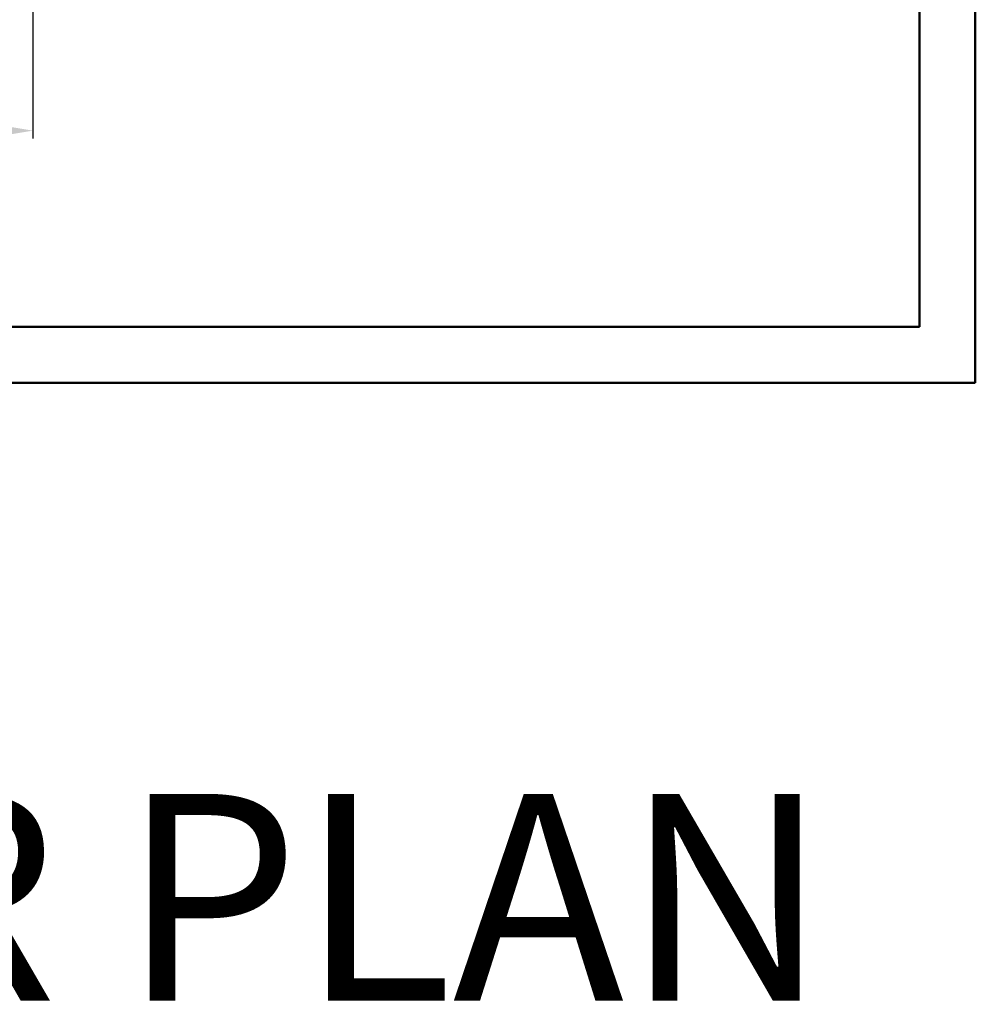
# Model space of a CAD drawing. Units: inches. Extents: x 116541 to 117938, y 135634 to 136328.
# Tile 6 of 9: x 117747 to 117902, y 135634 to 135793. Entities that reach past the tile are written whole.
import ezdxf

# ---------------------------------------------------------------- set-up
doc = ezdxf.new("R2010")
doc.units = ezdxf.units.IN
for name, color, linetype, lineweight in [('A-ANNO-DIMS', 2, 'Continuous', 18), ('A-ANNO-TEXT', 7, 'Continuous', 25), ('A-WALL', 7, 'Continuous', 50)]:
    doc.layers.add(name, color=color, linetype=linetype, lineweight=lineweight)
doc.styles.get("Standard").update_dxf_attribs({"font": 'arial.ttf'})
doc.dimstyles.new('ISO-25', dxfattribs={"dimtxt": 5, "dimasz": 4, "dimexe": 1.25, "dimexo": 0.625, "dimtad": 1, "dimdec": 3, "dimlunit": 3, "dimtxsty": 'Standard', "dimcen": 2.5, "dimadec": 0, "dimazin": 0, "dimtfac": 1, "dimtdec": 3, "dimtmove": 0, "dimatfit": 3, "dimfxl": 1, "dimarcsym": 0})

# ---------------------------------------------------------------- blocks, each defined once
blk = doc.blocks.new('*D50')
at = {"layer": 'A-ANNO-DIMS', "color": 0, "lineweight": -2, "transparency": 16777216}
for p, q in [((117487.52, 135796.88), (117487.52, 135773.9)), ((117749.52, 135796.88), (117749.52, 135773.9)), ((117491.52, 135775.15), (117745.52, 135775.15))]:
    blk.add_line(p, q, dxfattribs=at)
at = {"layer": 'A-ANNO-DIMS', "color": 0, "transparency": 16777216}
for points in [[(117491.52, 135775.82), (117491.52, 135774.49), (117487.52, 135775.15)], [(117745.52, 135775.82), (117745.52, 135774.49), (117749.52, 135775.15)]]:
    blk.add_solid(points, dxfattribs=at)
at = {"layer": 'Defpoints', "color": 0, "transparency": 16777216}
for p in [(117487.52, 135797.5), (117749.52, 135797.5), (117749.52, 135775.15)]:
    blk.add_point(p, dxfattribs=at)
at = {"layer": 'A-ANNO-DIMS', "color": 0, "transparency": 16777216, "insert": (117618.52, 135778.33), "char_height": 5, "attachment_point": 5}
blk.add_mtext('21\'-10"', dxfattribs=at)

msp = doc.modelspace()

# ---------------------------------------------------------------- linework, layer by layer
at = {"layer": 'A-WALL'}
for p, q in [((117901.5209, 136286.5034), (117901.5209, 135734.5034)), ((117892.5209, 136244.5034), (117892.5209, 135750.0323)), ((117892.5209, 135743.5034), (117892.5209, 135750.0323)), ((117698.4977, 135743.5034), (117892.5209, 135743.5034)), ((117454.5209, 135734.5034), (117871.5209, 135734.5034)), ((117871.5209, 135734.5034), (117901.5209, 135734.5034))]:
    msp.add_line(p, q, dxfattribs=at)

# ---------------------------------------------------------------- texts
at = {"layer": 'A-ANNO-TEXT'}
msp.add_text('FIRST FLOOR PLAN', height=33.340721, dxfattribs=at).set_placement((117475.5022, 135634.8462))

# ---------------------------------------------------------------- dimensions: what is measured, and where the dimension line sits
at = {"layer": 'A-ANNO-DIMS'}
dim = msp.add_linear_dim(base=(117749.5209, 135775.1534), p1=(117487.5209, 135797.5034), p2=(117749.5209, 135797.5034), dimstyle='ISO-25', override={"dimclrd": 0, "dimclre": 0, "dimclrt": 0}, dxfattribs=at)
dim.commit()
dim.dimension.update_dxf_attribs({"geometry": '*D50', "text_midpoint": (117618.5209, 135778.3313)})

doc.saveas('drawing.dxf')
